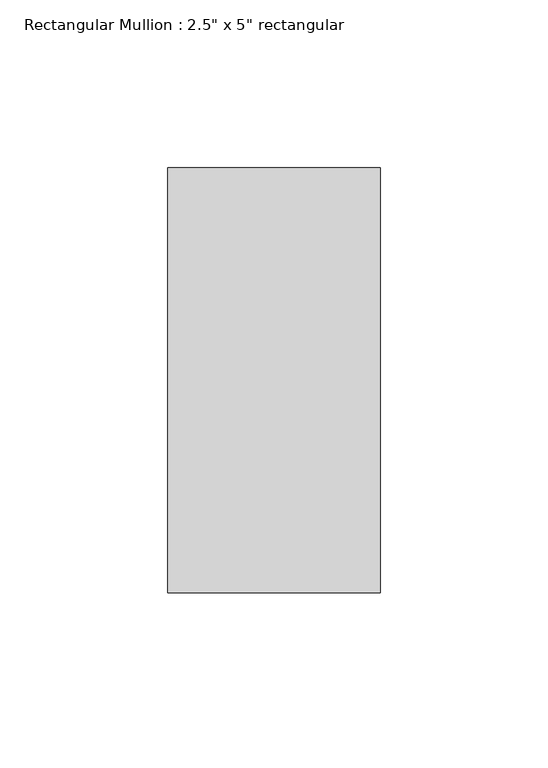
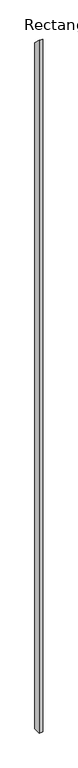
"""IFC4 building model written with IfcOpenShell, lengths in millimetres: member geometry."""

from ifc_helpers import new_model, si_unit, frame, origin, place, context, project, spatial, polyline, outline, extrude, source, transform, mapped, element, save


def member_fed80fbc(model_context):
    return source(origin(), model_context, "Body", "SweptSolid", [
        extrude(outline(polyline([(-63.5, 63.5), (63.5, -63.5), (63.5, -12757.6283072), (-63.5, -12757.6283072), (-63.5, 63.5)])), frame((-63.5, 0.0, 0.0), z_axis=(1.0, 0.0, 0.0), x_axis=(0.0, 1.0, 0.0)), (0.0, 0.0, 1.0), 63.5),
    ])


if __name__ == "__main__":
    model = new_model("IFC4")
    model_context = context("Model", 3, world=origin())
    ifc_project = project(units=[si_unit("LENGTHUNIT", "METRE", prefix="MILLI")], contexts=[model_context])
    site = spatial("IfcSite", under=ifc_project)
    building = spatial("IfcBuilding", under=site)
    placement = place(None, origin())
    member_shape = member_fed80fbc(model_context)
    element("IfcMember", 1, ObjectType="Rectangular Mullion : 2.5\" x 5\" rectangular", at=placement, inside=building, context=model_context, shape_type="MappedRepresentation", body=[
        mapped(member_shape, transform((0.0, 0.0, 0.0), x_axis=(1.0, 0.0, 0.0), y_axis=(0.0, 1.0, 0.0), z_axis=(0.0, 0.0, 1.0))),
    ])
    save(model, "model.ifc")

# Revit data of these elements
# Type "Rectangular Mullion : 2.5\" x 5\" rectangular"
#   built-in parameter 1007304 = 0.416667 (stored number, unit not read)
#   built-in parameter 1007301 = 0.104167 (stored number, unit not read)
#   built-in parameter 1007300 = 0.104167 (stored number, unit not read)
# Element 1 (IfcMember, "Rectangular Mullion : 2.5\" x 5\" rectangular")
#   Materials on its faces: "Aluminum"
# Materials
#   "Aluminum": class "Metal", colour RGB 247 247 247, transparency 0, Description = "Aluminum 6061", Cost = 0
